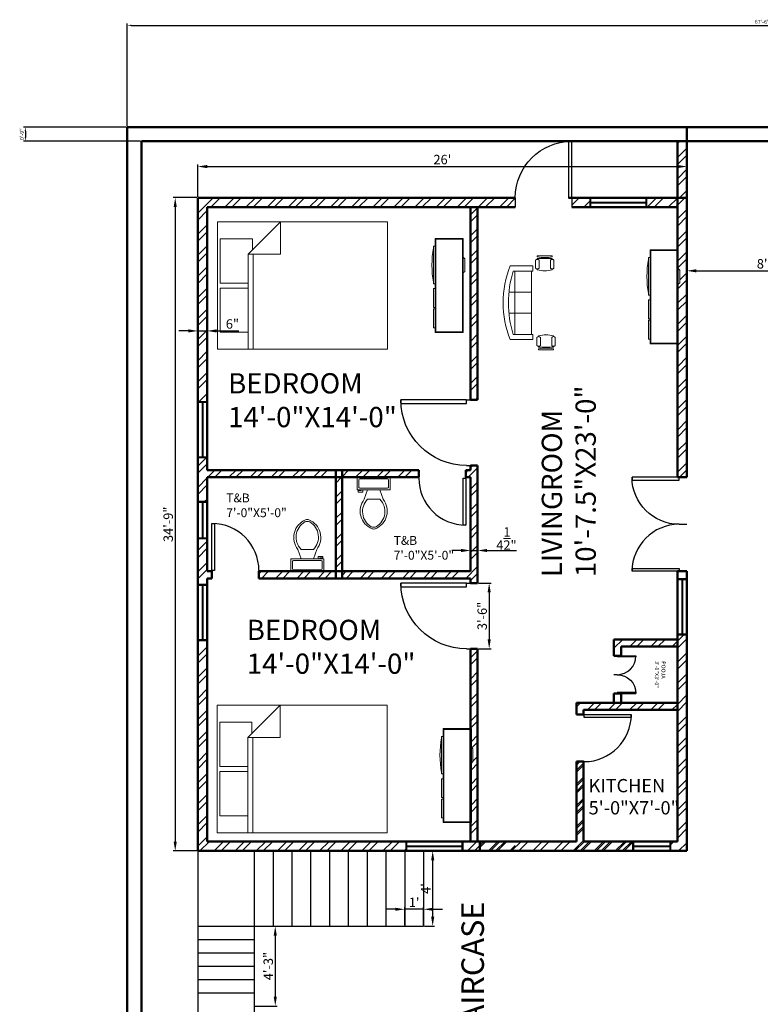
# Model space of a CAD drawing. Units: inches. Extents: x -12550 to 6516, y 1273 to 18700.
# Tile 14 of 19: x 4339 to 4811, y 1958 to 2587. Entities that reach past the tile are written whole.
import ezdxf

# ---------------------------------------------------------------- set-up
doc = ezdxf.new("R2010")
doc.units = ezdxf.units.IN
for name, color, linetype, lineweight in [('A-ANNO-DIMS', 2, 'Continuous', 18), ('A-AREA-IDEN', 1, 'Continuous', 18), ('A-DOOR', 5, 'Continuous', 25), ('A-FLOR-STRS', 6, 'Continuous', 25), ('A-FURN', 8, 'Continuous', 18), ('A-GLAZ', 3, 'Continuous', 25), ('A-WALL', 7, 'Continuous', 50), ('A-WALL-PATT', 8, 'Continuous', 13)]:
    doc.layers.add(name, color=color, linetype=linetype, lineweight=lineweight)
doc.styles.get("Standard").update_dxf_attribs({"font": 'arial.ttf'})
doc.dimstyles.new('ISO-25', dxfattribs={"dimtxt": 2.5, "dimasz": 2.5, "dimexe": 1.25, "dimexo": 0.625, "dimtad": 1, "dimlunit": 4, "dimtxsty": 'Standard', "dimcen": 2.5, "dimadec": 0, "dimazin": 0, "dimtfac": 1, "dimtmove": 0, "dimatfit": 3, "dimfxl": 1, "dimarcsym": 0})
pattern_1 = [(45, (2434.941, 0), (-6.735192, 6.735192), []), (45, (2439.432, 0), (-6.735192, 6.735192), [])]
pattern_2 = [(45, (2434.941, 567), (-6.735192, 6.735192), []), (45, (2439.432, 567), (-6.735192, 6.735192), [])]

# ---------------------------------------------------------------- blocks, each defined once
blk = doc.blocks.new('*U2')
for p, q in [((0, 0), (0, -5)), ((30, 0), (30, -5))]:
    blk.add_line(p, q)
blk.add_lwpolyline([(0, 0), (0, 30), (1.75, 30), (1.75, 0)], close=True)
blk.add_arc((0, 0), 30, 0, 90)
blk = doc.blocks.new('Bed - Queen')
for p, q in [((0, -80.00003), (0, 0)), ((0, 0), (59.99999, 0)), ((59.99999, 0), (59.99999, -80.00003)), ((7.99999, -1.2), (28.79998, -1.2)), ((7.99999, -14.4), (7.99999, -1.2)), ((28.79998, -1.2), (28.79998, -14.4)), ((31.19999, -1.2), (51.99999, -1.2)), ((31.19999, -14.4), (31.19999, -1.2)), ((51.99999, -1.2), (51.99999, -16.4)), ((0, -14.4), (44.8, -14.4)), ((44.8, -16.8), (0, -16.8)), ((59.99999, -29.6), (44.8, -14.4)), ((44.8, -14.4), (44.8, -29.6)), ((51.99999, -16.4), (46.79936, -16.4)), ((44.8, -29.6), (59.99999, -29.6)), ((59.99999, -80.00003), (0, -80.00003))]:
    blk.add_line(p, q)
blk = doc.blocks.new('Toilet - top')
for p, q in [((9.5, -6), (9.5, -2)), ((-10, -8.5), (-8, -8.5)), ((-10, -9.5), (-10, -8.5)), ((-7, -9.5), (-10, -9.5)), ((-8, -8.5), (-8, -8)), ((-7, -8), (-7, -9.5)), ((-4, -8), (-6, -14)), ((4, -8), (6, -14)), ((4, -14), (-4, -14))]:
    blk.add_line(p, q)
blk.add_lwpolyline([(10.5, -8), (10.5, 0), (-10.5, 0), (-10.5, -8)], close=True)
for points in [[(-9.5, -2), (-9.5, -6)], [(8.5, -1), (-8.5, -1)], [(-8.5, -7), (8.5, -7)]]:
    blk.add_lwpolyline(points)
for centre, radius, start, end in [((-8.62, -1.88), 0.884, 81.8699, 188.1301), ((-8.62, -6.12), 0.884, 171.8699, 278.1301), ((8.62, -1.88), 0.884, 351.8699, 98.1301), ((8.62, -6.12), 0.884, 261.8699, 8.1301), ((3.52, -21.58), 12.17, 141.46911, 247.97143), ((4.2, -21.82), 11.33, 136.36773, 238.94682), ((-3.52, -21.58), 12.17, 292.02843, 38.53071), ((-4.2, -21.82), 11.33, 301.05301, 43.63209), ((0, -27.88), 4, 245.73182, 294.26817), ((0, -29), 4, 254.86053, 285.13947)]:
    blk.add_arc(centre, radius, start, end)
blk = doc.blocks.new('Entertainment Center')
for p, q in [((-4, 0), (-5, -1)), ((4, 0), (-4, 0)), ((5, -1), (4, 0)), ((-17, -19), (-17, -1)), ((-17, -1), (43, -1)), ((-16.5, -18.5), (-16.5, -1.5)), ((-16.5, -1.5), (42.5, -1.5)), ((42.5, -1.5), (42.5, -18.5)), ((43, -1), (43, -19)), ((42.5, -18.5), (-16.5, -18.5)), ((43, -19), (-17, -19)), ((-12, -20), (-12, -19)), ((12, -20), (-12, -20)), ((12, -19), (12, -20)), ((15, -20), (15, -19)), ((27, -20), (15, -20)), ((27, -19), (27, -20)), ((28, -20), (28, -19)), ((40, -20), (28, -20)), ((40, -19), (40, -20))]:
    blk.add_line(p, q)
blk.add_arc((0, 40), 61, 259.6111, 280.3889)
blk = doc.blocks.new('Sofa - Roundback 7 ft.')
for p, q in [((-12.00002, -32.4421), (-12.00003, -6.5971)), ((11.99997, -32.4421), (11.99998, -6.5971)), ((-36.000027, -34), (-36.000027, -11.4696)), ((-35.999844, -13.3819), (35.9998, -13.3819)), ((35.99998, -34), (35.99998, -11.4696)), ((-36.000027, -32.4421), (35.99998, -32.4421))]:
    blk.add_line(p, q)
for points in [[(-36.000027, -34), (-42.000027, -34), (-42.000027, -8)], [(41.99998, -8), (41.99998, -34), (35.99998, -34)]]:
    blk.add_lwpolyline(points)
for centre, radius, start, end in [((0, -114.25), 114.25, 68.43141, 111.5686), ((-0.00001, -127.1968), 121.1968, 72.72033, 107.2797)]:
    blk.add_arc(centre, radius, start, end)
blk = doc.blocks.new('Chair - Desk')
for p, q in [((-8.5, 0), (-8.5, -1)), ((-8.5, 0), (8.5, 0)), ((8.5, 0), (8.5, -1)), ((-10.5, -5), (-10.5, -14)), ((-8.5, -3), (-8.5, -4)), ((-8.5, -3), (8.5, -3)), ((-6.5, -14), (-6.5, -5)), ((-2, -3), (-2, -1.9355)), ((2, -1.9576), (2, -3)), ((6.5, -5), (6.5, -14)), ((8.5, -3), (8.5, -4)), ((10.5, -14), (10.5, -5)), ((-8.5, -15), (-8.5, -16)), ((8.5, -15), (8.5, -16))]:
    blk.add_line(p, q)
for centre, radius, start, end in [((-8.5, -6.5), 2.5, 36.8699, 143.1301), ((0, 34.625), 36.625, 256.5803, 283.4197), ((8.5, -6.5), 2.5, 36.8699, 143.1301), ((-8.5, -12.5), 2.5, 216.8699, 323.1301), ((0, 19.625), 36.625, 256.5803, 283.4197), ((8.5, -12.5), 2.5, 216.8699, 323.1301)]:
    blk.add_arc(centre, radius, start, end)
blk = doc.blocks.new('*D37')
at = {"layer": 'A-ANNO-DIMS', "color": 0, "lineweight": -2, "transparency": 16777216}
for p, q in [((4452.63, 2388.03), (4452.63, 2389.43)), ((4458.63, 2388.03), (4458.63, 2389.43)), ((4446.63, 2388.18), (4440.63, 2388.18)), ((4452.63, 2388.18), (4458.63, 2388.18)), ((4464.63, 2388.18), (4478.81, 2388.18))]:
    blk.add_line(p, q, dxfattribs=at)
at = {"layer": 'A-ANNO-DIMS', "color": 0, "transparency": 16777216}
for points in [[(4446.63, 2389.18), (4446.63, 2387.18), (4452.63, 2388.18)], [(4464.63, 2389.18), (4464.63, 2387.18), (4458.63, 2388.18)]]:
    blk.add_solid(points, dxfattribs=at)
at = {"layer": 'Defpoints', "color": 0, "transparency": 16777216}
for p in [(4452.63, 2387.4), (4458.63, 2388.18), (4458.63, 2387.4)]:
    blk.add_point(p, dxfattribs=at)
at = {"layer": 'A-ANNO-DIMS', "color": 0, "transparency": 16777216, "insert": (4474.72, 2391.87), "char_height": 6, "attachment_point": 5}
blk.add_mtext('6"', dxfattribs=at)
blk = doc.blocks.new('*D38')
at = {"layer": 'A-ANNO-DIMS', "color": 0, "lineweight": -2, "transparency": 16777216}
for p, q in [((4626.63, 2251.78), (4626.63, 2246.78)), ((4631.13, 2251.78), (4631.13, 2246.78)), ((4620.63, 2248.03), (4614.63, 2248.03)), ((4626.63, 2248.03), (4631.13, 2248.03)), ((4637.13, 2248.03), (4655.89, 2248.03))]:
    blk.add_line(p, q, dxfattribs=at)
at = {"layer": 'A-ANNO-DIMS', "color": 0, "transparency": 16777216}
for points in [[(4620.63, 2249.03), (4620.63, 2247.03), (4626.63, 2248.03)], [(4637.13, 2249.03), (4637.13, 2247.03), (4631.13, 2248.03)]]:
    blk.add_solid(points, dxfattribs=at)
at = {"layer": 'Defpoints', "color": 0, "transparency": 16777216}
for p in [(4626.63, 2252.41), (4631.13, 2252.41), (4631.13, 2248.03)]:
    blk.add_point(p, dxfattribs=at)
at = {"layer": 'A-ANNO-DIMS', "color": 0, "transparency": 16777216, "insert": (4649.51, 2255.68), "char_height": 6, "attachment_point": 5}
blk.add_mtext('4{\\H1x;\\S1/2;}"', dxfattribs=at)
blk = doc.blocks.new('*D45')
at = {"layer": 'A-ANNO-DIMS', "color": 0, "lineweight": -2, "transparency": 16777216}
for p, q in [((4631.76, 2227.25), (4639.76, 2227.25)), ((4638.51, 2221.25), (4638.51, 2191.25)), ((4631.76, 2185.25), (4639.76, 2185.25))]:
    blk.add_line(p, q, dxfattribs=at)
at = {"layer": 'A-ANNO-DIMS', "color": 0, "transparency": 16777216}
for points in [[(4637.51, 2221.25), (4639.51, 2221.25), (4638.51, 2227.25)], [(4637.51, 2191.25), (4639.51, 2191.25), (4638.51, 2185.25)]]:
    blk.add_solid(points, dxfattribs=at)
at = {"layer": 'Defpoints', "color": 0, "transparency": 16777216}
for p in [(4631.13, 2227.25), (4631.13, 2185.25), (4638.51, 2185.25)]:
    blk.add_point(p, dxfattribs=at)
at = {"layer": 'A-ANNO-DIMS', "color": 0, "transparency": 16777216, "insert": (4634.82, 2206.25), "char_height": 6, "attachment_point": 5, "rotation": 90}
blk.add_mtext('3\'-6"', dxfattribs=at)
blk = doc.blocks.new('*D46')
at = {"layer": 'A-ANNO-DIMS', "color": 0, "lineweight": -2, "transparency": 16777216}
for p, q in [((4597.26, 2056.25), (4603.73, 2056.25)), ((4602.48, 2014.25), (4602.48, 2050.25)), ((4597.26, 2008.25), (4603.73, 2008.25))]:
    blk.add_line(p, q, dxfattribs=at)
at = {"layer": 'A-ANNO-DIMS', "color": 0, "transparency": 16777216}
for points in [[(4601.48, 2050.25), (4603.48, 2050.25), (4602.48, 2056.25)], [(4601.48, 2014.25), (4603.48, 2014.25), (4602.48, 2008.25)]]:
    blk.add_solid(points, dxfattribs=at)
at = {"layer": 'Defpoints', "color": 0, "transparency": 16777216}
for p in [(4596.63, 2056.25), (4602.48, 2056.25), (4596.63, 2008.25)]:
    blk.add_point(p, dxfattribs=at)
at = {"layer": 'A-ANNO-DIMS', "color": 0, "transparency": 16777216, "insert": (4598.86, 2032.25), "char_height": 6, "attachment_point": 5, "rotation": 90}
blk.add_mtext("4'", dxfattribs=at)
blk = doc.blocks.new('*D47')
at = {"layer": 'A-ANNO-DIMS', "color": 0, "lineweight": -2, "transparency": 16777216}
for p, q in [((4578.63, 2019.01), (4572.63, 2019.01)), ((4584.63, 2008.87), (4584.63, 2020.26)), ((4596.63, 2019.01), (4584.63, 2019.01)), ((4596.63, 2008.87), (4596.63, 2020.26)), ((4602.63, 2019.01), (4608.63, 2019.01))]:
    blk.add_line(p, q, dxfattribs=at)
at = {"layer": 'A-ANNO-DIMS', "color": 0, "transparency": 16777216}
for points in [[(4578.63, 2020.01), (4578.63, 2018.01), (4584.63, 2019.01)], [(4602.63, 2020.01), (4602.63, 2018.01), (4596.63, 2019.01)]]:
    blk.add_solid(points, dxfattribs=at)
at = {"layer": 'Defpoints', "color": 0, "transparency": 16777216}
for p in [(4584.63, 2019.01), (4584.63, 2008.25), (4596.63, 2008.25)]:
    blk.add_point(p, dxfattribs=at)
at = {"layer": 'A-ANNO-DIMS', "color": 0, "transparency": 16777216, "insert": (4590.63, 2022.65), "char_height": 6, "attachment_point": 5}
blk.add_mtext("1'", dxfattribs=at)
blk = doc.blocks.new('*D48')
at = {"layer": 'A-ANNO-DIMS', "color": 0, "lineweight": -2, "transparency": 16777216}
for p, q in [((4489.26, 2008.25), (4503.3, 2008.25)), ((4502.05, 2002.25), (4502.05, 1963.25)), ((4489.26, 1957.25), (4503.3, 1957.25))]:
    blk.add_line(p, q, dxfattribs=at)
at = {"layer": 'A-ANNO-DIMS', "color": 0, "transparency": 16777216}
for points in [[(4501.05, 2002.25), (4503.05, 2002.25), (4502.05, 2008.25)], [(4501.05, 1963.25), (4503.05, 1963.25), (4502.05, 1957.25)]]:
    blk.add_solid(points, dxfattribs=at)
at = {"layer": 'Defpoints', "color": 0, "transparency": 16777216}
for p in [(4488.63, 2008.25), (4488.63, 1957.25), (4502.05, 1957.25)]:
    blk.add_point(p, dxfattribs=at)
at = {"layer": 'A-ANNO-DIMS', "color": 0, "transparency": 16777216, "insert": (4498.36, 1982.75), "char_height": 6, "attachment_point": 5, "rotation": 90}
blk.add_mtext('4\'-3"', dxfattribs=at)
blk = doc.blocks.new('*D41')
at = {"layer": 'A-ANNO-DIMS', "color": 0, "lineweight": -2, "transparency": 16777216}
for p, q in [((4452.01, 2473.25), (4436.97, 2473.25)), ((4438.22, 2467.25), (4438.22, 2062.25)), ((4452.01, 2056.25), (4436.97, 2056.25))]:
    blk.add_line(p, q, dxfattribs=at)
at = {"layer": 'A-ANNO-DIMS', "color": 0, "transparency": 16777216}
for points in [[(4437.22, 2467.25), (4439.22, 2467.25), (4438.22, 2473.25)], [(4437.22, 2062.25), (4439.22, 2062.25), (4438.22, 2056.25)]]:
    blk.add_solid(points, dxfattribs=at)
at = {"layer": 'Defpoints', "color": 0, "transparency": 16777216}
for p in [(4452.63, 2473.25), (4438.22, 2056.25), (4452.63, 2056.25)]:
    blk.add_point(p, dxfattribs=at)
at = {"layer": 'A-ANNO-DIMS', "color": 0, "transparency": 16777216, "insert": (4434.53, 2264.75), "char_height": 6, "attachment_point": 5, "rotation": 90}
blk.add_mtext('34\'-9"', dxfattribs=at)
blk = doc.blocks.new('*D44')
at = {"layer": 'A-ANNO-DIMS', "color": 0, "lineweight": -2, "transparency": 16777216}
for p, q in [((4452.63, 2473.87), (4452.63, 2494.36)), ((4458.63, 2493.11), (4758.63, 2493.11)), ((4764.63, 2473.87), (4764.63, 2494.36))]:
    blk.add_line(p, q, dxfattribs=at)
at = {"layer": 'A-ANNO-DIMS', "color": 0, "transparency": 16777216}
for points in [[(4458.63, 2494.11), (4458.63, 2492.11), (4452.63, 2493.11)], [(4758.63, 2494.11), (4758.63, 2492.11), (4764.63, 2493.11)]]:
    blk.add_solid(points, dxfattribs=at)
at = {"layer": 'Defpoints', "color": 0, "transparency": 16777216}
for p in [(4764.63, 2493.11), (4452.63, 2473.25), (4764.63, 2473.25)]:
    blk.add_point(p, dxfattribs=at)
at = {"layer": 'A-ANNO-DIMS', "color": 0, "transparency": 16777216, "insert": (4608.63, 2496.8), "char_height": 6, "attachment_point": 5}
blk.add_mtext("26'", dxfattribs=at)
blk = doc.blocks.new('*D39')
at = {"layer": 'A-ANNO-DIMS', "color": 0, "lineweight": -2, "transparency": 16777216}
for p, q in [((4764.63, 2407.12), (4764.63, 2427.81)), ((4770.63, 2426.56), (4854.63, 2426.56)), ((4860.63, 2407.12), (4860.63, 2427.81))]:
    blk.add_line(p, q, dxfattribs=at)
at = {"layer": 'A-ANNO-DIMS', "color": 0, "transparency": 16777216}
for points in [[(4770.63, 2427.56), (4770.63, 2425.56), (4764.63, 2426.56)], [(4854.63, 2427.56), (4854.63, 2425.56), (4860.63, 2426.56)]]:
    blk.add_solid(points, dxfattribs=at)
at = {"layer": 'Defpoints', "color": 0, "transparency": 16777216}
for p in [(4860.63, 2426.56), (4764.63, 2406.5), (4860.63, 2406.5)]:
    blk.add_point(p, dxfattribs=at)
at = {"layer": 'A-ANNO-DIMS', "color": 0, "transparency": 16777216, "insert": (4812.63, 2430.25), "char_height": 6, "attachment_point": 5}
blk.add_mtext("8'", dxfattribs=at)
blk = doc.blocks.new('WIN-3FT')
for p, q in [((0, 0), (0, 6)), ((0, 6), (36.02, 6)), ((36.02, 0), (0, 0)), ((0.5, 0), (0.5, 6)), ((35.52, 3.2), (0.5, 3.2)), ((35.52, 2.8), (0.5, 2.8)), ((35.52, 6), (35.52, 0)), ((36.02, 6), (36.02, 0))]:
    blk.add_line(p, q)
blk = doc.blocks.new('WIN-2FT')
for p, q in [((0, 0), (0, 24.02)), ((0, 24.02), (6, 24.02)), ((0, 23.52), (6, 23.52)), ((2.8, 0.5), (2.8, 23.52)), ((3.2, 0.5), (3.2, 23.52)), ((6, 24.02), (6, 0)), ((6, 0.5), (0, 0.5)), ((6, 0), (0, 0))]:
    blk.add_line(p, q)
blk = doc.blocks.new('*D112')
at = {"layer": 'A-ANNO-DIMS', "color": 0, "lineweight": -2, "transparency": 16777216}
for p, q in [((4407.63, 2518.87), (4407.63, 2584.5)), ((4410.13, 2583.25), (5215.13, 2583.25)), ((5217.63, 2518.87), (5217.63, 2584.5))]:
    blk.add_line(p, q, dxfattribs=at)
at = {"layer": 'A-ANNO-DIMS', "color": 0, "transparency": 16777216}
for points in [[(4410.13, 2583.66), (4410.13, 2582.83), (4407.63, 2583.25)], [(5215.13, 2583.66), (5215.13, 2582.83), (5217.63, 2583.25)]]:
    blk.add_solid(points, dxfattribs=at)
at = {"layer": 'Defpoints', "color": 0, "transparency": 16777216}
for p in [(5217.63, 2583.25), (4407.63, 2518.25), (5217.63, 2518.25)]:
    blk.add_point(p, dxfattribs=at)
at = {"layer": 'A-ANNO-DIMS', "color": 0, "transparency": 16777216, "insert": (4812.63, 2585.15), "char_height": 2.5, "attachment_point": 5}
blk.add_mtext('67\'-6"', dxfattribs=at)
blk = doc.blocks.new('*D120')
at = {"layer": 'A-ANNO-DIMS', "color": 0, "lineweight": -2, "transparency": 16777216}
for p, q in [((4407.01, 2518.25), (4341.38, 2518.25)), ((4342.63, 2515.75), (4342.63, 2511.75)), ((4416.01, 2509.25), (4341.38, 2509.25))]:
    blk.add_line(p, q, dxfattribs=at)
at = {"layer": 'A-ANNO-DIMS', "color": 0, "transparency": 16777216}
for points in [[(4342.21, 2515.75), (4343.05, 2515.75), (4342.63, 2518.25)], [(4342.21, 2511.75), (4343.05, 2511.75), (4342.63, 2509.25)]]:
    blk.add_solid(points, dxfattribs=at)
at = {"layer": 'Defpoints', "color": 0, "transparency": 16777216}
for p in [(4407.63, 2518.25), (4342.63, 2509.25), (4416.63, 2509.25)]:
    blk.add_point(p, dxfattribs=at)
at = {"layer": 'A-ANNO-DIMS', "color": 0, "transparency": 16777216, "insert": (4340.73, 2513.75), "char_height": 2.5, "attachment_point": 5, "rotation": 90}
blk.add_mtext('0\'-9"', dxfattribs=at)

msp = doc.modelspace()

# ---------------------------------------------------------------- hatches: boundary and pattern name
at = {"layer": 'A-WALL-PATT'}
h = msp.add_hatch(dxfattribs=at)
h.set_pattern_fill('ANSI32', color=256)
h.set_pattern_definition(pattern_1)
h.paths.add_polyline_path([(4764.63, 2509.247), (4758.63, 2509.247), (4758.63, 2473.247), (4764.63, 2473.247)])
h = msp.add_hatch(dxfattribs=at)
h.set_pattern_fill('ANSI32', color=256)
h.set_pattern_definition(pattern_2)
h.paths.add_polyline_path([(4458.63, 2467.247), (4632.63, 2467.247), (4632.63, 2473.247), (4452.63, 2473.247), (4452.63, 2343.138), (4458.63, 2343.138)])
h = msp.add_hatch(dxfattribs=at)
h.set_pattern_fill('ANSI32', color=256)
h.set_pattern_definition(pattern_2)
h.paths.add_polyline_path([(4691.13, 2473.247), (4691.13, 2467.247), (4702.882, 2467.247), (4702.882, 2473.247)])
h.paths.add_polyline_path([(4655.13, 2467.247), (4655.13, 2473.247), (4632.63, 2473.247), (4632.63, 2467.247)])
h = msp.add_hatch(dxfattribs=at)
h.set_pattern_fill('ANSI32', color=256)
h.set_pattern_definition(pattern_2)
h.paths.add_polyline_path([(4764.63, 2473.247), (4738.899, 2473.247), (4738.899, 2467.247), (4758.63, 2467.247), (4758.63, 2439.972), (4759.13, 2439.972), (4759.13, 2427.972), (4760.13, 2426.972), (4760.13, 2418.972), (4759.13, 2417.972), (4759.13, 2379.972), (4758.63, 2294.747), (4759.63, 2294.747), (4764.63, 2294.747)])
h = msp.add_hatch(dxfattribs=at)
h.set_pattern_fill('ANSI32', color=256)
h.set_pattern_definition(pattern_2)
h.paths.add_polyline_path([(4631.13, 2467.247), (4626.63, 2467.247), (4626.63, 2344.247), (4631.13, 2344.247)], flags=17)
h = msp.add_hatch(dxfattribs=at)
h.set_pattern_fill('ANSI32', color=256)
h.set_pattern_definition(pattern_2)
h.paths.add_polyline_path([(4540.63, 2299.247), (4458.63, 2299.247), (4458.63, 2307.121), (4452.63, 2307.121), (4452.63, 2279.466), (4458.63, 2279.466), (4458.63, 2294.747), (4540.63, 2294.747)])
h = msp.add_hatch(dxfattribs=at)
h.set_pattern_fill('ANSI32', color=256)
h.set_pattern_definition(pattern_2)
h.paths.add_polyline_path([(4631.13, 2302.247), (4626.63, 2302.247), (4626.63, 2299.247), (4623.63, 2299.247), (4623.63, 2294.747), (4626.63, 2294.747), (4626.63, 2234.747), (4544.63, 2234.747), (4544.63, 2230.247), (4626.63, 2230.247), (4626.63, 2227.247), (4631.13, 2227.247)])
h = msp.add_hatch(dxfattribs=at)
h.set_pattern_fill('ANSI32', color=256)
h.set_pattern_definition(pattern_2)
h.paths.add_polyline_path([(4544.63, 2294.747), (4540.63, 2294.747), (4540.63, 2234.747), (4544.63, 2234.747)])
h = msp.add_hatch(dxfattribs=at)
h.set_pattern_fill('ANSI32', color=256)
h.set_pattern_definition(pattern_2)
h.paths.add_polyline_path([(4593.63, 2299.247), (4544.63, 2299.247), (4544.63, 2294.747), (4593.63, 2294.747)], flags=17)
h = msp.add_hatch(dxfattribs=at)
h.set_pattern_fill('ANSI32', color=256)
h.set_pattern_definition(pattern_2)
h.paths.add_polyline_path([(4458.63, 2255.449), (4452.63, 2255.449), (4452.63, 2226.453), (4458.63, 2226.453), (4458.63, 2230.247), (4461.63, 2230.247), (4461.63, 2234.747), (4458.63, 2234.747)])
h = msp.add_hatch(dxfattribs=at)
h.set_pattern_fill('ANSI32', color=256)
h.set_pattern_definition(pattern_2)
h.paths.add_polyline_path([(4540.63, 2234.747), (4491.63, 2234.747), (4491.63, 2230.247), (4540.63, 2230.247)])
h = msp.add_hatch(dxfattribs=at)
h.set_pattern_fill('ANSI32', color=256)
h.set_pattern_definition(pattern_2)
h.paths.add_polyline_path([(4764.63, 2194.032), (4758.63, 2194.032), (4758.63, 2062.247), (4754.235, 2062.247), (4754.235, 2056.247), (4764.63, 2056.247)])
h = msp.add_hatch(dxfattribs=at)
h.set_pattern_fill('ANSI32', color=256)
h.set_pattern_definition(pattern_2)
h.paths.add_polyline_path([(4458.63, 2190.435), (4452.63, 2190.435), (4452.63, 2056.247), (4585.581, 2056.247), (4585.581, 2062.247), (4458.63, 2062.247)])
h = msp.add_hatch(dxfattribs=at)
h.set_pattern_fill('ANSI32', color=256)
h.set_pattern_definition(pattern_2)
h.paths.add_polyline_path([(4758.63, 2191.247), (4718.13, 2191.247), (4718.13, 2180.747), (4720.13, 2180.747), (4722.63, 2180.747), (4722.63, 2186.747), (4758.63, 2186.747)])
h = msp.add_hatch(dxfattribs=at)
h.set_pattern_fill('ANSI32', color=256)
h.set_pattern_definition(pattern_2)
h.paths.add_polyline_path([(4631.13, 2185.247), (4626.63, 2185.247), (4626.63, 2134.365), (4627.13, 2134.365), (4627.13, 2122.365), (4628.13, 2121.365), (4628.13, 2113.365), (4627.13, 2112.365), (4627.13, 2074.365), (4626.63, 2062.247), (4631.13, 2062.247)])
h = msp.add_hatch(dxfattribs=at)
h.set_pattern_fill('ANSI32', color=256)
h.set_pattern_definition(pattern_2)
h.paths.add_polyline_path([(4758.63, 2150.747), (4694.13, 2150.747), (4694.13, 2143.247), (4698.63, 2143.247), (4698.63, 2146.247), (4758.63, 2146.247)])
h = msp.add_hatch(dxfattribs=at)
h.set_pattern_fill('ANSI32', color=256)
h.set_pattern_definition(pattern_1)
h.paths.add_polyline_path([(4730.218, 2062.247), (4698.63, 2062.247), (4698.63, 2113.247), (4694.13, 2113.247), (4694.13, 2062.247), (4691.13, 2062.247), (4632.63, 2062.247), (4632.63, 2056.247), (4691.13, 2056.247), (4730.218, 2056.247)])
h = msp.add_hatch(dxfattribs=at)
h.set_pattern_fill('ANSI32', color=256)
h.set_pattern_definition(pattern_2)
h.paths.add_polyline_path([(4698.63, 2062.247), (4698.63, 2113.247), (4694.13, 2113.247), (4694.13, 2062.247), (4691.13, 2062.247), (4691.13, 2056.247), (4730.218, 2056.247), (4730.218, 2062.247)])
h = msp.add_hatch(dxfattribs=at)
h.set_pattern_fill('ANSI32', color=256)
h.set_pattern_definition(pattern_2)
h.paths.add_polyline_path([(4621.598, 2062.247), (4621.598, 2056.247), (4655.13, 2056.247), (4655.13, 2062.247)])

# ---------------------------------------------------------------- linework, layer by layer
at = {"layer": 'A-FLOR-STRS'}
for p, q in [((4632.63, 2056.247), (4452.63, 2056.247)), ((4452.63, 2056.247), (4452.63, 1906.247)), ((4488.63, 2056.247), (4488.63, 1906.247)), ((4500.63, 2056.247), (4500.63, 2008.247)), ((4512.63, 2056.247), (4512.63, 2008.247)), ((4524.63, 2056.247), (4524.63, 2008.247)), ((4536.63, 2056.247), (4536.63, 2008.247)), ((4548.63, 2056.247), (4548.63, 2008.247)), ((4560.63, 2056.247), (4560.63, 2008.247)), ((4572.63, 2056.247), (4572.63, 2008.247)), ((4584.63, 2056.247), (4584.63, 2008.247)), ((4596.63, 2056.247), (4596.63, 2008.247)), ((4452.63, 2008.247), (4596.63, 2008.247)), ((4452.63, 2008.247), (4596.63, 2008.247)), ((4452.63, 1999.747), (4488.63, 1999.747)), ((4452.63, 1991.247), (4488.63, 1991.247)), ((4452.63, 1982.747), (4488.63, 1982.747)), ((4452.63, 1974.247), (4488.63, 1974.247)), ((4452.63, 1965.747), (4488.63, 1965.747))]:
    msp.add_line(p, q, dxfattribs=at)
at = {"layer": 'A-WALL'}
for p, q in [((4407.63, 1444.247), (4407.63, 2518.247)), ((4407.63, 2518.247), (5217.63, 2518.247)), ((4764.63, 2294.747), (4764.63, 2518.247)), ((4416.63, 1453.247), (4416.63, 2509.247)), ((4416.63, 2509.247), (5208.63, 2509.247)), ((4989.03, 2509.247), (4689.03, 2509.247)), ((4758.63, 2294.747), (4758.63, 2509.247)), ((4655.13, 2473.247), (4452.63, 2473.247)), ((4452.63, 2068.324), (4452.63, 2473.247)), ((4764.63, 2473.247), (4689.03, 2473.247)), ((4655.13, 2467.247), (4458.63, 2467.247)), ((4458.63, 2299.247), (4458.63, 2467.247)), ((4626.63, 2344.247), (4626.63, 2467.247)), ((4631.13, 2344.247), (4631.13, 2467.247)), ((4758.63, 2467.247), (4691.13, 2467.247)), ((4631.13, 2344.247), (4626.63, 2344.247)), ((4626.63, 2299.247), (4626.63, 2302.247)), ((4626.63, 2299.247), (4626.63, 2302.247)), ((4626.63, 2302.247), (4631.13, 2302.247)), ((4631.13, 2227.247), (4631.13, 2302.247)), ((4593.63, 2299.247), (4458.63, 2299.247)), ((4593.63, 2294.747), (4458.63, 2294.747)), ((4458.63, 2234.747), (4458.63, 2294.747)), ((4540.63, 2230.247), (4540.63, 2299.247)), ((4544.63, 2230.247), (4544.63, 2299.247)), ((4593.63, 2294.747), (4593.63, 2299.247)), ((4626.63, 2299.247), (4623.63, 2299.247)), ((4626.63, 2299.247), (4623.63, 2299.247)), ((4623.63, 2299.247), (4623.63, 2294.747)), ((4626.63, 2294.747), (4623.63, 2294.747)), ((4626.63, 2234.747), (4626.63, 2294.747)), ((4764.63, 2294.747), (4758.63, 2294.747)), ((4461.63, 2234.747), (4458.63, 2234.747)), ((4461.63, 2230.247), (4461.63, 2234.747)), ((4626.63, 2234.747), (4491.63, 2234.747)), ((4491.63, 2234.747), (4626.63, 2234.747)), ((4491.63, 2234.747), (4491.63, 2230.247)), ((4764.63, 2234.747), (4758.63, 2234.747)), ((4758.63, 2062.247), (4758.63, 2234.747)), ((4764.63, 2056.247), (4764.63, 2234.747)), ((4461.63, 2230.247), (4458.63, 2230.247)), ((4458.63, 2062.247), (4458.63, 2230.247)), ((4458.63, 2230.247), (4461.63, 2230.247)), ((4626.63, 2230.247), (4491.63, 2230.247)), ((4626.63, 2227.247), (4626.63, 2230.247)), ((4631.13, 2227.247), (4626.63, 2227.247)), ((4631.13, 2230.247), (4631.13, 2227.247)), ((4758.63, 2191.247), (4718.13, 2191.247)), ((4718.13, 2180.747), (4718.13, 2191.247)), ((4626.63, 2062.247), (4626.63, 2185.247)), ((4626.63, 2185.247), (4631.13, 2185.247)), ((4631.13, 2062.247), (4631.13, 2185.247)), ((4758.63, 2186.747), (4722.63, 2186.747)), ((4722.63, 2180.747), (4722.63, 2186.747)), ((4718.13, 2180.747), (4722.63, 2180.747)), ((4718.13, 2150.747), (4718.13, 2156.747)), ((4722.63, 2156.747), (4718.13, 2156.747)), ((4722.63, 2150.747), (4722.63, 2156.747)), ((4722.63, 2150.747), (4722.63, 2156.747)), ((4758.63, 2150.747), (4694.13, 2150.747)), ((4694.13, 2143.247), (4694.13, 2150.747)), ((4718.13, 2150.747), (4718.13, 2155.747)), ((4698.63, 2143.247), (4694.13, 2143.247)), ((4758.63, 2146.247), (4698.63, 2146.247)), ((4698.63, 2143.247), (4698.63, 2146.247)), ((4698.63, 2146.247), (4698.63, 2143.247)), ((4694.13, 2062.247), (4694.13, 2113.247)), ((4694.13, 2113.247), (4698.63, 2113.247)), ((4698.63, 2062.247), (4698.63, 2113.247)), ((4452.63, 2056.247), (4452.63, 2068.324)), ((4691.13, 2062.247), (4458.63, 2062.247)), ((4655.13, 2062.247), (4631.13, 2062.247)), ((4632.63, 2056.247), (4632.63, 2062.247)), ((4694.13, 2062.247), (4691.13, 2062.247)), ((4694.13, 2062.247), (4691.13, 2062.247)), ((4758.63, 2062.247), (4698.63, 2062.247)), ((4691.13, 2056.247), (4452.63, 2056.247)), ((4764.63, 2056.247), (4691.13, 2056.247))]:
    msp.add_line(p, q, dxfattribs=at)

# ---------------------------------------------------------------- block references
at = {"layer": 'A-DOOR', "xscale": -1.199999999999999, "yscale": 1.199999999999999, "zscale": 1.199999999999999}
msp.add_blockref('*U2', (4691.13, 2473.247), dxfattribs=at)
at = {"layer": 'A-DOOR'}
for p, xscale, yscale, zscale, rotation in [((4624.13, 2344.247), -1.4, 1.4, 1.4, 90), ((4624.13, 2227.247), -1.4, 1.4, 1.4, 90), ((4720.13, 2180.747), 0.399999999999997, 0.399999999999997, 0.399999999999997, 270), ((4720.13, 2156.747), -0.399999999999997, 0.399999999999997, 0.399999999999997, 270)]:
    msp.add_blockref('*U2', p, dxfattribs=dict(at, xscale=xscale, yscale=yscale, zscale=zscale, rotation=rotation))
for p, rotation in [((4623.63, 2294.247), 180), ((4759.63, 2234.747), 90), ((4699.13, 2143.247), 270)]:
    msp.add_blockref('*U2', p, dxfattribs=dict(at, rotation=rotation))
at = {"layer": 'A-DOOR', "xscale": -1, "rotation": 90}
msp.add_blockref('*U2', (4759.63, 2294.747), dxfattribs=at)
at = {"layer": 'A-DOOR'}
msp.add_blockref('*U2', (4461.63, 2235.247), dxfattribs=at)
at = {"layer": 'A-FURN'}
for name, p, xscale, yscale, zscale, rotation in [('Bed - Queen', (4465.28, 2376.493), 1.354827908062564, 1.354827908062564, 1.354827908062564, 90), ('Sofa - Roundback 7 ft.', (4647.389, 2406.138), 0.5595223685495907, 0.5595223685495907, 0.5595223685495907, 90), ('Chair - Desk', (4674.829, 2376.138), 0.5595223685495907, 0.5595223685495907, 0.5595223685495907, 180), ('Bed - Queen', (4464.979, 2067.915), 1.354827908062564, 1.354827908062564, 1.354827908062564, 90)]:
    msp.add_blockref(name, p, dxfattribs=dict(at, xscale=xscale, yscale=yscale, zscale=zscale, rotation=rotation))
for name, p, rotation in [('Entertainment Center', (4622.971, 2430.204), 270), ('Entertainment Center', (4760.13, 2422.972), 270), ('Toilet - top', (4522.477, 2234.747), 180), ('Entertainment Center', (4628.13, 2117.365), 270)]:
    msp.add_blockref(name, p, dxfattribs=dict(at, rotation=rotation))
at = {"layer": 'A-FURN', "xscale": 0.5595223685495907, "yscale": 0.5595223685495907, "zscale": 0.5595223685495907}
msp.add_blockref('Chair - Desk', (4673.975, 2436.122), dxfattribs=at)
at = {"layer": 'A-FURN'}
msp.add_blockref('Toilet - top', (4564.841, 2294.747), dxfattribs=at)
at = {"layer": 'A-GLAZ'}
for name, p, rotation in [('WIN-3FT', (4738.899, 2473.247), 180), ('WIN-3FT', (4458.63, 2307.121), 90.00000000000188), ('WIN-2FT', (4458.63, 2279.467), 180), ('WIN-3FT', (4458.63, 2190.436), 90.0000000000021), ('WIN-3FT', (4764.63, 2194.032), 89.99999999999625), ('WIN-3FT', (4621.598, 2062.247), 180), ('WIN-2FT', (4730.218, 2062.247), 270.0000000000005)]:
    msp.add_blockref(name, p, dxfattribs=dict(at, rotation=rotation))

# ---------------------------------------------------------------- texts
at = {"layer": 'A-AREA-IDEN', "char_height": 12.93169, "attachment_point": 1}
for insert in [(4471.967, 2361.217), (4483.848, 2203.812)]:
    msp.add_mtext('BEDROOM\\P14\'-0"X14\'-0"', dxfattribs=dict(at, insert=insert))
at = {"layer": 'A-AREA-IDEN', "insert": (4672.036, 2231.034), "char_height": 12.93169, "attachment_point": 1, "rotation": 90}
msp.add_mtext('LIVINGROOM\\P10\'-7.5"X23\'-0"', dxfattribs=at)
at = {"layer": 'A-AREA-IDEN', "attachment_point": 1}
for s, width, gutter_width, insert, char_height in [('T&B\\P7\'-0"X5\'-0"', 4.19569, 28.328, (4470.806, 2284.416), 5.66556), ('T&B\\P7\'-0"X5\'-0"', 4.19569, 28.328, (4577.568, 2257.282), 5.66556), ('KITCHEN\\P5\'-0"X7\'-0"', 1.29487, 42.422, (4701.952, 2102.176), 8.48435)]:
    msp.add_mtext_dynamic_manual_height_columns(s, width=width, gutter_width=gutter_width, heights=[0], dxfattribs=dict(at, insert=insert, char_height=char_height))
for s, width, gutter_width, insert, char_height, rotation in [('POOJA\\P3\'-0"X3\'-0"', 0.78585, 12.5, (4751.006, 2177.304), 2.5, 269.183853), ('STAIRCASE', 2.19144, 71.795, (4620.807, 1922.837), 14.3589, 90)]:
    msp.add_mtext_dynamic_manual_height_columns(s, width=width, gutter_width=gutter_width, heights=[0], dxfattribs=dict(at, insert=insert, char_height=char_height, rotation=rotation))

# ---------------------------------------------------------------- dimensions: what is measured, and where the dimension line sits
at = {"layer": 'A-ANNO-DIMS'}
for base, p1, p2, override, picture, middle in [((5217.63, 2583.247), (4407.63, 2518.247), (5217.63, 2518.247), {"dimdec": 1, "dimlfac": 1, "dimrnd": 0, "dimzin": 1, "dimdsep": 46, "dimlunit": 4, "dimfrac": 2}, '*D112', (4812.63, 2585.149)), ((4764.63, 2493.114), (4452.63, 2473.247), (4764.63, 2473.247), {"dimtxt": 6, "dimasz": 6, "dimclrd": 0, "dimclre": 0, "dimclrt": 0}, '*D44', (4608.63, 2496.802)), ((4860.63, 2426.562), (4764.63, 2406.497), (4860.63, 2406.497), {"dimtxt": 6, "dimasz": 6, "dimclrd": 0, "dimclre": 0, "dimclrt": 0}, '*D39', (4812.63, 2430.25)), ((4458.63, 2388.182), (4452.63, 2387.405), (4458.63, 2387.405), {"dimtxt": 6, "dimasz": 6, "dimclrd": 0, "dimclre": 0, "dimclrt": 0}, '*D37', (4474.72, 2391.871)), ((4631.13, 2248.034), (4626.63, 2252.406), (4631.13, 2252.406), {"dimtxt": 6, "dimasz": 6, "dimclrd": 0, "dimclre": 0, "dimclrt": 0}, '*D38', (4649.512, 2255.683)), ((4584.63, 2019.012), (4596.63, 2008.247), (4584.63, 2008.247), {"dimtxt": 6, "dimasz": 6, "dimclrd": 0, "dimclre": 0, "dimclrt": 0}, '*D47', (4590.63, 2022.65))]:
    dim = msp.add_linear_dim(base=base, p1=p1, p2=p2, dimstyle='ISO-25', override=override, dxfattribs=at)
    dim.commit()
    dim.dimension.update_dxf_attribs({"geometry": picture, "text_midpoint": middle})
for base, p1, p2, override, picture, middle in [((4342.63, 2509.247), (4407.63, 2518.247), (4416.63, 2509.247), {"dimdec": 1, "dimlfac": 1, "dimrnd": 0, "dimzin": 1, "dimdsep": 46, "dimlunit": 4, "dimfrac": 2}, '*D120', (4340.729, 2513.747)), ((4438.222, 2056.247), (4452.63, 2473.247), (4452.63, 2056.247), {"dimtxt": 6, "dimasz": 6, "dimclrd": 0, "dimclre": 0, "dimclrt": 0}, '*D41', (4434.531, 2264.747)), ((4638.514, 2185.247), (4631.13, 2227.247), (4631.13, 2185.247), {"dimtxt": 6, "dimasz": 6, "dimclrd": 0, "dimclre": 0, "dimclrt": 0}, '*D45', (4634.823, 2206.247)), ((4602.483, 2056.247), (4596.63, 2008.247), (4596.63, 2056.247), {"dimtxt": 6, "dimasz": 6, "dimclrd": 0, "dimclre": 0, "dimclrt": 0}, '*D46', (4598.858, 2032.247)), ((4502.052, 1957.247), (4488.63, 2008.247), (4488.63, 1957.247), {"dimtxt": 6, "dimasz": 6, "dimclrd": 0, "dimclre": 0, "dimclrt": 0}, '*D48', (4498.362, 1982.747))]:
    dim = msp.add_linear_dim(base=base, p1=p1, p2=p2, angle=90, dimstyle='ISO-25', override=override, dxfattribs=at)
    dim.commit()
    dim.dimension.update_dxf_attribs({"geometry": picture, "text_midpoint": middle})

doc.saveas('drawing.dxf')
